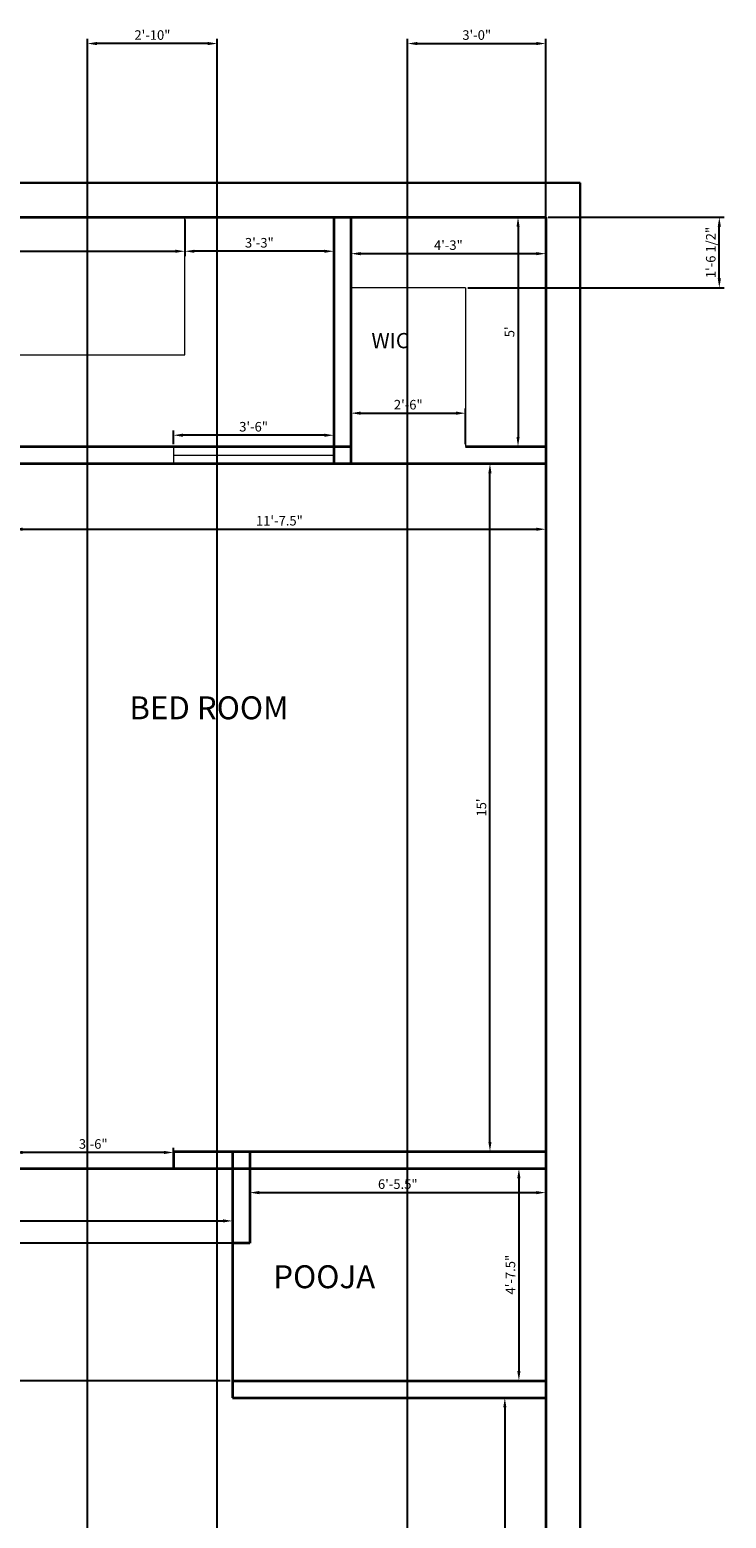
# Model space of a CAD drawing. Units: inches. Extents: x 2279 to 2719, y 394 to 1171.
# Tile 3 of 3: x 2537 to 2719, y 779 to 1169. Entities that reach past the tile are written whole.
import ezdxf

# ---------------------------------------------------------------- set-up
doc = ezdxf.new("R2010")
doc.units = ezdxf.units.IN
for name, color, linetype, lineweight in [('A-ANNO-DIMS', 2, 'Continuous', 13), ('A-AREA-IDEN', 7, 'Continuous', 25), ('A-FLOR-CASE', 8, 'Continuous', 18), ('A-FLOR-OPEN', 4, 'Continuous', 18), ('A-GLAZ', 4, 'Continuous', 18), ('A-WALL', 7, 'Continuous', 35), ('C-PROP', 7, 'Continuous', 30)]:
    doc.layers.add(name, color=color, linetype=linetype, lineweight=lineweight)
doc.styles.get("Standard").update_dxf_attribs({"font": 'arial.ttf'})
doc.dimstyles.new('ISO-25', dxfattribs={"dimtxt": 2.5, "dimasz": 2.5, "dimexe": 1.25, "dimexo": 0.625, "dimtad": 1, "dimdec": 1, "dimlunit": 3, "dimtxsty": 'Standard', "dimcen": 2.5, "dimadec": 0, "dimazin": 0, "dimtfac": 1, "dimtdec": 1, "dimtmove": 0, "dimatfit": 3, "dimfxl": 1, "dimarcsym": 0})

# ---------------------------------------------------------------- blocks, each defined once
blk = doc.blocks.new('*D4')
at = {"layer": 'A-ANNO-DIMS', "color": 0, "lineweight": -2, "transparency": 16777216}
for p, q in [((2577.64, 1118.83), (2577.64, 1109.29)), ((2616.64, 1118.83), (2616.64, 1109.29)), ((2614.14, 1110.54), (2580.14, 1110.54))]:
    blk.add_line(p, q, dxfattribs=at)
at = {"layer": 'A-ANNO-DIMS', "color": 0, "transparency": 16777216}
for points in [[(2580.14, 1110.95), (2580.14, 1110.12), (2577.64, 1110.54)], [(2614.14, 1110.95), (2614.14, 1110.12), (2616.64, 1110.54)]]:
    blk.add_solid(points, dxfattribs=at)
at = {"layer": 'Defpoints', "color": 0, "transparency": 16777216}
for p in [(2577.64, 1119.45), (2616.64, 1119.45), (2577.64, 1110.54)]:
    blk.add_point(p, dxfattribs=at)
at = {"layer": 'A-ANNO-DIMS', "color": 0, "transparency": 16777216, "insert": (2597.14, 1112.44), "char_height": 2.5, "attachment_point": 5}
blk.add_mtext('3\'-3"', dxfattribs=at)
blk = doc.blocks.new('*D5')
at = {"layer": 'A-ANNO-DIMS', "color": 0, "lineweight": -2, "transparency": 16777216}
for p, q in [((2466.64, 1118.83), (2466.64, 1109.29)), ((2577.64, 1118.83), (2577.64, 1109.29)), ((2469.14, 1110.54), (2575.14, 1110.54))]:
    blk.add_line(p, q, dxfattribs=at)
at = {"layer": 'A-ANNO-DIMS', "color": 0, "transparency": 16777216}
for points in [[(2469.14, 1110.95), (2469.14, 1110.12), (2466.64, 1110.54)], [(2575.14, 1110.95), (2575.14, 1110.12), (2577.64, 1110.54)]]:
    blk.add_solid(points, dxfattribs=at)
at = {"layer": 'Defpoints', "color": 0, "transparency": 16777216}
for p in [(2466.64, 1119.45), (2577.64, 1119.45), (2577.64, 1110.54)]:
    blk.add_point(p, dxfattribs=at)
at = {"layer": 'A-ANNO-DIMS', "color": 0, "transparency": 16777216, "insert": (2522.14, 1112.44), "char_height": 2.5, "attachment_point": 5}
blk.add_mtext('9\'-3"', dxfattribs=at)
blk = doc.blocks.new('*D6')
at = {"layer": 'A-ANNO-DIMS', "color": 0, "lineweight": -2, "transparency": 16777216}
for p, q in [((2621.14, 1118.83), (2621.14, 1108.66)), ((2672.14, 1118.83), (2672.14, 1108.66)), ((2623.64, 1109.91), (2669.64, 1109.91))]:
    blk.add_line(p, q, dxfattribs=at)
at = {"layer": 'A-ANNO-DIMS', "color": 0, "transparency": 16777216}
for points in [[(2623.64, 1110.33), (2623.64, 1109.49), (2621.14, 1109.91)], [(2669.64, 1110.33), (2669.64, 1109.49), (2672.14, 1109.91)]]:
    blk.add_solid(points, dxfattribs=at)
at = {"layer": 'Defpoints', "color": 0, "transparency": 16777216}
for p in [(2621.14, 1119.45), (2672.14, 1119.45), (2672.14, 1109.91)]:
    blk.add_point(p, dxfattribs=at)
at = {"layer": 'A-ANNO-DIMS', "color": 0, "transparency": 16777216, "insert": (2646.64, 1111.81), "char_height": 2.5, "attachment_point": 5}
blk.add_mtext('4\'-3"', dxfattribs=at)
blk = doc.blocks.new('*D7')
at = {"layer": 'A-ANNO-DIMS', "color": 0, "lineweight": -2, "transparency": 16777216}
for p, q in [((2621.14, 1060.08), (2621.14, 1069.41)), ((2623.64, 1068.16), (2648.64, 1068.16)), ((2651.14, 1060.08), (2651.14, 1069.41))]:
    blk.add_line(p, q, dxfattribs=at)
at = {"layer": 'A-ANNO-DIMS', "color": 0, "transparency": 16777216}
for points in [[(2623.64, 1068.58), (2623.64, 1067.75), (2621.14, 1068.16)], [(2648.64, 1068.58), (2648.64, 1067.75), (2651.14, 1068.16)]]:
    blk.add_solid(points, dxfattribs=at)
at = {"layer": 'Defpoints', "color": 0, "transparency": 16777216}
for p in [(2651.14, 1068.16), (2621.14, 1059.45), (2651.14, 1059.45)]:
    blk.add_point(p, dxfattribs=at)
at = {"layer": 'A-ANNO-DIMS', "color": 0, "transparency": 16777216, "insert": (2636.14, 1070.06), "char_height": 2.5, "attachment_point": 5}
blk.add_mtext('2\'-6"', dxfattribs=at)
blk = doc.blocks.new('*D8')
at = {"layer": 'A-ANNO-DIMS', "color": 0, "lineweight": -2, "transparency": 16777216}
for p, q in [((2671.52, 1119.45), (2663.63, 1119.45)), ((2664.88, 1116.95), (2664.88, 1061.95)), ((2671.52, 1059.45), (2663.63, 1059.45))]:
    blk.add_line(p, q, dxfattribs=at)
at = {"layer": 'A-ANNO-DIMS', "color": 0, "transparency": 16777216}
for points in [[(2664.47, 1116.95), (2665.3, 1116.95), (2664.88, 1119.45)], [(2664.47, 1061.95), (2665.3, 1061.95), (2664.88, 1059.45)]]:
    blk.add_solid(points, dxfattribs=at)
at = {"layer": 'Defpoints', "color": 0, "transparency": 16777216}
for p in [(2672.14, 1119.45), (2664.88, 1059.45), (2672.14, 1059.45)]:
    blk.add_point(p, dxfattribs=at)
at = {"layer": 'A-ANNO-DIMS', "color": 0, "transparency": 16777216, "insert": (2662.99, 1089.45), "char_height": 2.5, "attachment_point": 5, "rotation": 90}
blk.add_mtext("5'", dxfattribs=at)
blk = doc.blocks.new('*D16')
at = {"layer": 'A-ANNO-DIMS', "color": 0, "lineweight": -2, "transparency": 16777216}
for p, q in [((2532.64, 1054.33), (2532.64, 1036.54)), ((2672.14, 1054.33), (2672.14, 1036.54)), ((2535.14, 1037.79), (2669.64, 1037.79))]:
    blk.add_line(p, q, dxfattribs=at)
at = {"layer": 'A-ANNO-DIMS', "color": 0, "transparency": 16777216}
for points in [[(2535.14, 1038.21), (2535.14, 1037.37), (2532.64, 1037.79)], [(2669.64, 1038.21), (2669.64, 1037.37), (2672.14, 1037.79)]]:
    blk.add_solid(points, dxfattribs=at)
at = {"layer": 'Defpoints', "color": 0, "transparency": 16777216}
for p in [(2532.64, 1054.95), (2672.14, 1054.95), (2672.14, 1037.79)]:
    blk.add_point(p, dxfattribs=at)
at = {"layer": 'A-ANNO-DIMS', "color": 0, "transparency": 16777216, "insert": (2602.39, 1039.69), "char_height": 2.5, "attachment_point": 5}
blk.add_mtext('11\'-7.5"', dxfattribs=at)
blk = doc.blocks.new('*D17')
at = {"layer": 'A-ANNO-DIMS', "color": 0, "lineweight": -2, "transparency": 16777216}
for p, q in [((2671.52, 1054.95), (2656.28, 1054.95)), ((2657.53, 877.45), (2657.53, 1052.45)), ((2671.52, 874.95), (2656.28, 874.95))]:
    blk.add_line(p, q, dxfattribs=at)
at = {"layer": 'A-ANNO-DIMS', "color": 0, "transparency": 16777216}
for points in [[(2657.11, 1052.45), (2657.94, 1052.45), (2657.53, 1054.95)], [(2657.11, 877.45), (2657.94, 877.45), (2657.53, 874.95)]]:
    blk.add_solid(points, dxfattribs=at)
at = {"layer": 'Defpoints', "color": 0, "transparency": 16777216}
for p in [(2657.53, 1054.95), (2672.14, 1054.95), (2672.14, 874.95)]:
    blk.add_point(p, dxfattribs=at)
at = {"layer": 'A-ANNO-DIMS', "color": 0, "transparency": 16777216, "insert": (2655.62, 964.95), "char_height": 2.5, "attachment_point": 5, "rotation": 90}
blk.add_mtext("15'", dxfattribs=at)
blk = doc.blocks.new('*D31')
at = {"layer": 'A-ANNO-DIMS', "color": 0, "lineweight": -2, "transparency": 16777216}
for p, q in [((2671.52, 870.45), (2663.85, 870.45)), ((2665.1, 867.95), (2665.1, 817.45)), ((2671.52, 814.95), (2663.85, 814.95))]:
    blk.add_line(p, q, dxfattribs=at)
at = {"layer": 'A-ANNO-DIMS', "color": 0, "transparency": 16777216}
for points in [[(2664.69, 867.95), (2665.52, 867.95), (2665.1, 870.45)], [(2664.69, 817.45), (2665.52, 817.45), (2665.1, 814.95)]]:
    blk.add_solid(points, dxfattribs=at)
at = {"layer": 'Defpoints', "color": 0, "transparency": 16777216}
for p in [(2672.14, 870.45), (2665.1, 814.95), (2672.14, 814.95)]:
    blk.add_point(p, dxfattribs=at)
at = {"layer": 'A-ANNO-DIMS', "color": 0, "transparency": 16777216, "insert": (2663.21, 842.7), "char_height": 2.5, "attachment_point": 5, "rotation": 90}
blk.add_mtext('4\'-7.5"', dxfattribs=at)
blk = doc.blocks.new('*D32')
at = {"layer": 'A-ANNO-DIMS', "color": 0, "lineweight": -2, "transparency": 16777216}
for p, q in [((2594.64, 869.83), (2594.64, 862.92)), ((2672.14, 869.83), (2672.14, 862.92)), ((2597.14, 864.17), (2669.64, 864.17))]:
    blk.add_line(p, q, dxfattribs=at)
at = {"layer": 'A-ANNO-DIMS', "color": 0, "transparency": 16777216}
for points in [[(2597.14, 864.59), (2597.14, 863.75), (2594.64, 864.17)], [(2669.64, 864.59), (2669.64, 863.75), (2672.14, 864.17)]]:
    blk.add_solid(points, dxfattribs=at)
at = {"layer": 'Defpoints', "color": 0, "transparency": 16777216}
for p in [(2594.64, 870.45), (2672.14, 870.45), (2672.14, 864.17)]:
    blk.add_point(p, dxfattribs=at)
at = {"layer": 'A-ANNO-DIMS', "color": 0, "transparency": 16777216, "insert": (2633.39, 866.07), "char_height": 2.5, "attachment_point": 5}
blk.add_mtext('6\'-5.5"', dxfattribs=at)
blk = doc.blocks.new('*D34')
at = {"layer": 'A-ANNO-DIMS', "color": 0, "lineweight": -2, "transparency": 16777216}
for p, q in [((2422.14, 850.08), (2422.14, 858.01)), ((2590.14, 850.08), (2590.14, 858.01)), ((2424.64, 856.76), (2587.64, 856.76))]:
    blk.add_line(p, q, dxfattribs=at)
at = {"layer": 'A-ANNO-DIMS', "color": 0, "transparency": 16777216}
for points in [[(2424.64, 857.18), (2424.64, 856.35), (2422.14, 856.76)], [(2587.64, 857.18), (2587.64, 856.35), (2590.14, 856.76)]]:
    blk.add_solid(points, dxfattribs=at)
at = {"layer": 'Defpoints', "color": 0, "transparency": 16777216}
for p in [(2590.14, 856.76), (2422.14, 849.45), (2590.14, 849.45)]:
    blk.add_point(p, dxfattribs=at)
at = {"layer": 'A-ANNO-DIMS', "color": 0, "transparency": 16777216, "insert": (2506.14, 858.64), "char_height": 2.5, "attachment_point": 5}
blk.add_mtext("14'", dxfattribs=at)
blk = doc.blocks.new('*U37')
for p, q in [((0, 100), (0, 0)), ((900, 100), (900, 0)), ((0, 50), (900, 50))]:
    blk.add_line(p, q)
blk = doc.blocks.new('*D41')
at = {"layer": 'A-ANNO-DIMS', "color": 0, "lineweight": -2, "transparency": 16777216}
for p, q in [((2574.64, 1060.08), (2574.64, 1063.64)), ((2616.64, 1060.08), (2616.64, 1063.64)), ((2614.14, 1062.39), (2577.14, 1062.39))]:
    blk.add_line(p, q, dxfattribs=at)
at = {"layer": 'A-ANNO-DIMS', "color": 0, "transparency": 16777216}
for points in [[(2577.14, 1062.81), (2577.14, 1061.97), (2574.64, 1062.39)], [(2614.14, 1062.81), (2614.14, 1061.97), (2616.64, 1062.39)]]:
    blk.add_solid(points, dxfattribs=at)
at = {"layer": 'Defpoints', "color": 0, "transparency": 16777216}
for p in [(2574.64, 1062.39), (2574.64, 1059.45), (2616.64, 1059.45)]:
    blk.add_point(p, dxfattribs=at)
at = {"layer": 'A-ANNO-DIMS', "color": 0, "transparency": 16777216, "insert": (2595.64, 1064.29), "char_height": 2.5, "attachment_point": 5}
blk.add_mtext('3\'-6"', dxfattribs=at)
blk = doc.blocks.new('*D43')
at = {"layer": 'A-ANNO-DIMS', "color": 0, "lineweight": -2, "transparency": 16777216}
for p, q in [((2532.64, 871.08), (2532.64, 875.93)), ((2572.14, 874.68), (2535.14, 874.68)), ((2574.64, 871.08), (2574.64, 875.93))]:
    blk.add_line(p, q, dxfattribs=at)
at = {"layer": 'A-ANNO-DIMS', "color": 0, "transparency": 16777216}
for points in [[(2535.14, 875.1), (2535.14, 874.26), (2532.64, 874.68)], [(2572.14, 875.1), (2572.14, 874.26), (2574.64, 874.68)]]:
    blk.add_solid(points, dxfattribs=at)
at = {"layer": 'Defpoints', "color": 0, "transparency": 16777216}
for p in [(2532.64, 874.68), (2532.64, 870.45), (2574.64, 870.45)]:
    blk.add_point(p, dxfattribs=at)
at = {"layer": 'A-ANNO-DIMS', "color": 0, "transparency": 16777216, "insert": (2553.64, 876.58), "char_height": 2.5, "attachment_point": 5}
blk.add_mtext('3\'-6"', dxfattribs=at)
blk = doc.blocks.new('*D47')
at = {"layer": 'A-ANNO-DIMS', "color": 0, "lineweight": -2, "transparency": 16777216}
for p, q in [((2671.52, 810.45), (2660.17, 810.45)), ((2661.42, 807.95), (2661.42, 713.95)), ((2671.52, 711.45), (2660.17, 711.45))]:
    blk.add_line(p, q, dxfattribs=at)
at = {"layer": 'A-ANNO-DIMS', "color": 0, "transparency": 16777216}
for points in [[(2661.01, 807.95), (2661.84, 807.95), (2661.42, 810.45)], [(2661.01, 713.95), (2661.84, 713.95), (2661.42, 711.45)]]:
    blk.add_solid(points, dxfattribs=at)
at = {"layer": 'Defpoints', "color": 0, "transparency": 16777216}
for p in [(2672.14, 810.45), (2661.42, 711.45), (2672.14, 711.45)]:
    blk.add_point(p, dxfattribs=at)
at = {"layer": 'A-ANNO-DIMS', "color": 0, "transparency": 16777216, "insert": (2659.52, 760.95), "char_height": 2.5, "attachment_point": 5, "rotation": 90}
blk.add_mtext('8\'-3"', dxfattribs=at)
blk = doc.blocks.new('*D53')
at = {"layer": 'A-ANNO-DIMS', "color": 0, "lineweight": -2, "transparency": 16777216}
for p, q in [((2552.14, 703.08), (2552.14, 1166.15)), ((2583.64, 1164.9), (2554.64, 1164.9)), ((2586.14, 623.28), (2586.14, 1166.15))]:
    blk.add_line(p, q, dxfattribs=at)
at = {"layer": 'A-ANNO-DIMS', "color": 0, "transparency": 16777216}
for points in [[(2554.64, 1165.32), (2554.64, 1164.48), (2552.14, 1164.9)], [(2583.64, 1165.32), (2583.64, 1164.48), (2586.14, 1164.9)]]:
    blk.add_solid(points, dxfattribs=at)
at = {"layer": 'Defpoints', "color": 0, "transparency": 16777216}
for p in [(2552.14, 1164.9), (2552.14, 702.45), (2586.14, 622.65)]:
    blk.add_point(p, dxfattribs=at)
at = {"layer": 'A-ANNO-DIMS', "color": 0, "transparency": 16777216, "insert": (2569.14, 1166.8), "char_height": 2.5, "attachment_point": 5}
blk.add_mtext('2\'-10"', dxfattribs=at)
blk = doc.blocks.new('*D55')
at = {"layer": 'A-ANNO-DIMS', "color": 0, "lineweight": -2, "transparency": 16777216}
for p, q in [((2635.98, 509.17), (2635.98, 1166.15)), ((2638.48, 1164.9), (2669.64, 1164.9)), ((2672.14, 442.08), (2672.14, 1166.15))]:
    blk.add_line(p, q, dxfattribs=at)
at = {"layer": 'A-ANNO-DIMS', "color": 0, "transparency": 16777216}
for points in [[(2638.48, 1165.32), (2638.48, 1164.48), (2635.98, 1164.9)], [(2669.64, 1165.32), (2669.64, 1164.48), (2672.14, 1164.9)]]:
    blk.add_solid(points, dxfattribs=at)
at = {"layer": 'Defpoints', "color": 0, "transparency": 16777216}
for p in [(2672.14, 1164.9), (2635.98, 508.54), (2672.14, 441.45)]:
    blk.add_point(p, dxfattribs=at)
at = {"layer": 'A-ANNO-DIMS', "color": 0, "transparency": 16777216, "insert": (2654.06, 1166.8), "char_height": 2.5, "attachment_point": 5}
blk.add_mtext('3\'-0"', dxfattribs=at)
blk = doc.blocks.new('*D60')
at = {"layer": 'A-ANNO-DIMS', "color": 0, "lineweight": -2, "transparency": 16777216}
for p, q in [((2672.77, 1119.45), (2718.84, 1119.45)), ((2717.59, 1103.47), (2717.59, 1116.95)), ((2651.77, 1100.97), (2718.84, 1100.97))]:
    blk.add_line(p, q, dxfattribs=at)
at = {"layer": 'A-ANNO-DIMS', "color": 0, "transparency": 16777216}
for points in [[(2717.17, 1116.95), (2718.01, 1116.95), (2717.59, 1119.45)], [(2717.17, 1103.47), (2718.01, 1103.47), (2717.59, 1100.97)]]:
    blk.add_solid(points, dxfattribs=at)
at = {"layer": 'Defpoints', "color": 0, "transparency": 16777216}
for p in [(2672.14, 1119.45), (2717.59, 1119.45), (2651.14, 1100.97)]:
    blk.add_point(p, dxfattribs=at)
at = {"layer": 'A-ANNO-DIMS', "color": 0, "transparency": 16777216, "insert": (2715.67, 1110.21), "char_height": 2.5, "attachment_point": 5, "rotation": 90}
blk.add_mtext('1\'-6 1/2"', dxfattribs=at)
blk = doc.blocks.new('*D62')
at = {"layer": 'A-ANNO-DIMS', "color": 0, "lineweight": -2, "transparency": 16777216}
for p, q in [((2594.02, 850.95), (2283.44, 850.95)), ((2284.69, 848.45), (2284.69, 817.45)), ((2589.52, 814.95), (2283.44, 814.95))]:
    blk.add_line(p, q, dxfattribs=at)
at = {"layer": 'A-ANNO-DIMS', "color": 0, "transparency": 16777216}
for points in [[(2284.27, 848.45), (2285.11, 848.45), (2284.69, 850.95)], [(2284.27, 817.45), (2285.11, 817.45), (2284.69, 814.95)]]:
    blk.add_solid(points, dxfattribs=at)
at = {"layer": 'Defpoints', "color": 0, "transparency": 16777216}
for p in [(2594.64, 850.95), (2284.69, 814.95), (2590.14, 814.95)]:
    blk.add_point(p, dxfattribs=at)
at = {"layer": 'A-ANNO-DIMS', "color": 0, "transparency": 16777216, "insert": (2282.79, 832.95), "char_height": 2.5, "attachment_point": 5, "rotation": 90}
blk.add_mtext('3\'-0"', dxfattribs=at)

msp = doc.modelspace()

# ---------------------------------------------------------------- linework, layer by layer
at = {"layer": 'A-FLOR-CASE'}
for q in [(2621.14, 1100.97), (2651.14, 1059.45)]:
    msp.add_line((2651.14, 1100.97), q, dxfattribs=at)
at = {"layer": 'A-FLOR-OPEN'}
for p, q in [((2577.64, 1083.45), (2577.64, 1119.45)), ((2466.64, 1083.45), (2577.64, 1083.45))]:
    msp.add_line(p, q, dxfattribs=at)
at = {"layer": 'A-GLAZ'}
msp.add_line((2574.64, 1059.45), (2574.64, 1054.95), dxfattribs=at)
at = {"layer": 'A-WALL'}
for p, q in [((2330.14, 1119.45), (2672.14, 1119.45)), ((2616.64, 1119.45), (2616.64, 1054.95)), ((2621.14, 1119.45), (2621.14, 1054.95)), ((2672.14, 1119.45), (2672.14, 441.45)), ((2427.64, 1059.45), (2621.14, 1059.45)), ((2651.14, 1059.45), (2672.14, 1059.45)), ((2505.64, 1054.95), (2672.14, 1054.95)), ((2574.64, 874.95), (2574.64, 870.45)), ((2574.64, 874.95), (2672.14, 874.95)), ((2590.14, 874.95), (2590.14, 810.45)), ((2594.64, 874.95), (2594.64, 850.95)), ((2469.64, 870.45), (2672.14, 870.45)), ((2594.64, 850.95), (2590.14, 850.95)), ((2590.14, 814.95), (2672.14, 814.95)), ((2590.14, 810.45), (2672.14, 810.45))]:
    msp.add_line(p, q, dxfattribs=at)
at = {"layer": 'C-PROP'}
for p, q in [((2321.14, 1128.45), (2681.14, 1128.45)), ((2681.14, 1128.45), (2681.14, 432.45))]:
    msp.add_line(p, q, dxfattribs=at)

# ---------------------------------------------------------------- block references
at = {"layer": 'A-GLAZ', "xscale": 0.0466666666666665, "yscale": 0.0466666666666665, "zscale": 0.0466666666666665}
msp.add_blockref('*U37', (2574.64, 1054.87), dxfattribs=at)

# ---------------------------------------------------------------- texts
at = {"layer": 'A-AREA-IDEN'}
for s, height, p in [('WIC', 4, (2626.49, 1085.15)), ('BED ROOM', 6, (2563.11, 988.05)), ('POOJA', 6, (2600.79, 839.15))]:
    msp.add_text(s, height=height, dxfattribs=at).set_placement(p)

# ---------------------------------------------------------------- dimensions: what is measured, and where the dimension line sits
at = {"layer": 'A-ANNO-DIMS'}
for base, p1, p2, override, picture, middle in [((2552.14, 1164.9), (2586.14, 622.65), (2552.14, 702.45), {"dimdec": 1, "dimlfac": 1, "dimrnd": 0, "dimzin": 1, "dimdsep": 46, "dimlunit": 4, "dimfrac": 2}, '*D53', (2569.14, 1166.8)), ((2672.14, 1164.9), (2635.98, 508.54), (2672.14, 441.45), {"dimdec": 1, "dimlfac": 1, "dimrnd": 0, "dimzin": 1, "dimdsep": 46, "dimlunit": 4, "dimfrac": 2}, '*D55', (2654.06, 1166.8)), ((2577.64, 1110.54), (2466.64, 1119.45), (2577.64, 1119.45), {"dimclrd": 0, "dimclre": 0, "dimclrt": 0}, '*D5', (2522.14, 1112.44)), ((2577.64, 1110.54), (2616.64, 1119.45), (2577.64, 1119.45), {"dimclrd": 0, "dimclre": 0, "dimclrt": 0}, '*D4', (2597.14, 1112.44)), ((2672.14, 1109.91), (2621.14, 1119.45), (2672.14, 1119.45), {"dimclrd": 0, "dimclre": 0, "dimclrt": 0}, '*D6', (2646.64, 1111.81)), ((2651.14, 1068.16), (2621.14, 1059.45), (2651.14, 1059.45), {"dimclrd": 0, "dimclre": 0, "dimclrt": 0}, '*D7', (2636.14, 1070.06)), ((2574.64, 1062.39), (2616.64, 1059.45), (2574.64, 1059.45), {"dimclrd": 0, "dimclre": 0, "dimclrt": 0}, '*D41', (2595.64, 1064.29)), ((2672.14, 1037.79), (2532.64, 1054.95), (2672.14, 1054.95), {"dimclrd": 0, "dimclre": 0, "dimclrt": 0}, '*D16', (2602.39, 1039.69)), ((2532.64, 874.68), (2574.64, 870.45), (2532.64, 870.45), {"dimclrd": 0, "dimclre": 0, "dimclrt": 0}, '*D43', (2553.64, 876.58)), ((2672.14, 864.17), (2594.64, 870.45), (2672.14, 870.45), {"dimclrd": 0, "dimclre": 0, "dimclrt": 0}, '*D32', (2633.39, 866.07)), ((2590.14, 856.76), (2422.14, 849.45), (2590.14, 849.45), {"dimclrd": 0, "dimclre": 0, "dimclrt": 0}, '*D34', (2506.14, 858.64))]:
    dim = msp.add_linear_dim(base=base, p1=p1, p2=p2, dimstyle='ISO-25', override=override, dxfattribs=at)
    dim.commit()
    dim.dimension.update_dxf_attribs({"geometry": picture, "text_midpoint": middle})
for base, p1, p2, override, picture, middle in [((2717.59, 1119.45), (2651.14, 1100.97), (2672.14, 1119.45), {"dimdec": 1, "dimlfac": 1, "dimrnd": 0, "dimzin": 1, "dimdsep": 46, "dimlunit": 4, "dimfrac": 2}, '*D60', (2715.67, 1110.21)), ((2664.88, 1059.45), (2672.14, 1119.45), (2672.14, 1059.45), {"dimclrd": 0, "dimclre": 0, "dimclrt": 0}, '*D8', (2662.99, 1089.45)), ((2657.53, 1054.95), (2672.14, 874.95), (2672.14, 1054.95), {"dimclrd": 0, "dimclre": 0, "dimclrt": 0}, '*D17', (2655.62, 964.95)), ((2665.1, 814.95), (2672.14, 870.45), (2672.14, 814.95), {"dimclrd": 0, "dimclre": 0, "dimclrt": 0}, '*D31', (2663.21, 842.7)), ((2284.69, 814.95), (2594.64, 850.95), (2590.14, 814.95), {"dimdec": 1, "dimlfac": 1, "dimrnd": 0, "dimzin": 1, "dimdsep": 46, "dimlunit": 4, "dimfrac": 2}, '*D62', (2282.79, 832.95)), ((2661.42, 711.45), (2672.14, 810.45), (2672.14, 711.45), {"dimclrd": 0, "dimclre": 0, "dimclrt": 0}, '*D47', (2659.52, 760.95))]:
    dim = msp.add_linear_dim(base=base, p1=p1, p2=p2, angle=90, dimstyle='ISO-25', override=override, dxfattribs=at)
    dim.commit()
    dim.dimension.update_dxf_attribs({"geometry": picture, "text_midpoint": middle})

doc.saveas('drawing.dxf')
